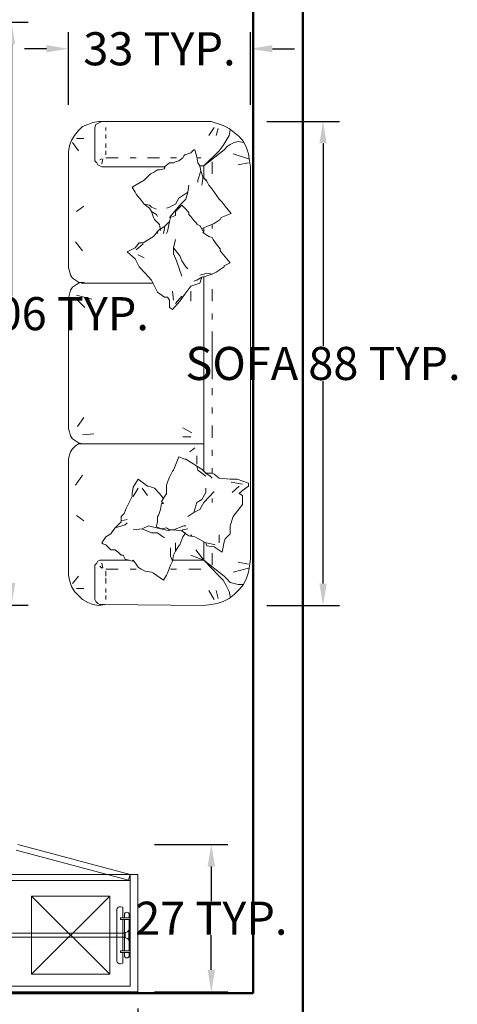
# Model space of a CAD drawing. Units: inches. Extents: x -466983 to 1020, y 324 to 318697.
# Tile 96 of 97: x 940 to 1020, y 827 to 1006. Entities that reach past the tile are written whole.
import ezdxf

# ---------------------------------------------------------------- set-up
doc = ezdxf.new("R2010")
doc.units = ezdxf.units.IN
doc.header["$MEASUREMENT"] = 0
for name, color, linetype, lineweight in [('A-ANNO-DIMS', 2, 'Continuous', 18), ('A-FURN', 8, 'Continuous', 18), ('A-WALL', 7, 'Continuous', 50)]:
    doc.layers.add(name, color=color, linetype=linetype, lineweight=lineweight)
doc.styles.get("Standard").update_dxf_attribs({"font": 'arial.ttf'})
doc.dimstyles.get("Standard").update_dxf_attribs({"dimtxt": 6, "dimasz": 4, "dimexe": 3, "dimexo": 3, "dimgap": 0.09, "dimtad": 0, "dimtih": 1, "dimtoh": 1, "dimdec": 1, "dimzin": 0, "dimdsep": 46, "dimlunit": 3, "dimtxsty": 'Standard', "dimcen": 0.09, "dimadec": 0, "dimazin": 0, "dimtfac": 1, "dimtdec": 1, "dimtofl": 0, "dimtmove": 0, "dimatfit": 3, "dimfxl": 1, "dimtolj": 1, "dimtzin": 0, "dimarcsym": 0})

# ---------------------------------------------------------------- blocks, each defined once
blk = doc.blocks.new('Wardrobe')
for p, q in [((2738.89, 1517.19, 0), (2738.89, 1543.9, 0)), ((2738.89, 1543.9, 0), (2850.18, 1543.9, 0)), ((2848.4, 1542.57, 0), (2740.67, 1542.57, 0)), ((2740.67, 1542.57, 0), (2740.67, 1517.19, 0)), ((2740.94, 1532.1, 0), (2740.67, 1532.1, 0)), ((2740.94, 1532.1, 0), (2740.67, 1532.1, 0)), ((2740.94, 1532.1, 0), (2740.94, 1529.88, 0)), ((2740.94, 1532.1, 0), (2740.94, 1529.88, 0)), ((2741.78, 1531.61, 0), (2741.78, 1530.37, 0)), ((2741.78, 1531.45, 0), (2792.53, 1531.45, 0)), ((2740.94, 1529.88, 0), (2740.67, 1529.88, 0)), ((2740.94, 1529.88, 0), (2740.67, 1529.88, 0)), ((2741.78, 1530.56, 0), (2792.53, 1530.56, 0)), ((2848.4, 1518.53, 0), (2740.67, 1518.53, 0)), ((2740.67, 1517.19, 0), (2741.02, 1518.48, 0)), ((2741.02, 1518.48, 0), (2766.6, 1511.65, 0)), ((2740.67, 1517.19, 0), (2738.89, 1517.19, 0)), ((2848.4, 1517.19, 0), (2740.67, 1517.19, 0)), ((2766.26, 1510.37, 0), (2740.67, 1517.19, 0))]:
    blk.add_line(p, q)
at = {"ltscale": 0.106667}
for p, q in [((2745.32, 1522.09, 0), (2763.13, 1539.9, 0)), ((2745.32, 1522.09, 0), (2745.32, 1539.9, 0)), ((2745.32, 1539.9, 0), (2763.13, 1539.9, 0)), ((2763.13, 1522.09, 0), (2745.32, 1539.9, 0)), ((2763.13, 1539.9, 0), (2763.13, 1522.09, 0)), ((2763.13, 1522.09, 0), (2745.32, 1522.09, 0))]:
    blk.add_line(p, q, dxfattribs=at)
at = {"ltscale": 0.02}
for p, q in [((2742.34, 1537.37, 0), (2742.84, 1537.5, 0)), ((2740.87, 1534.92, 0), (2740.87, 1535.62, 0)), ((2741.99, 1535.62, 0), (2741.99, 1534.92, 0)), ((2742.34, 1534.92, 0), (2742.34, 1537.37, 0)), ((2743.67, 1536.85, 0), (2743.67, 1525.18, 0)), ((2740.67, 1534.92, 0), (2742.84, 1534.92, 0)), ((2742.84, 1534.53, 0), (2740.67, 1534.53, 0)), ((2740.87, 1527.45, 0), (2740.87, 1534.53, 0)), ((2741.99, 1534.53, 0), (2741.99, 1527.45, 0)), ((2742.34, 1527.45, 0), (2742.34, 1534.53, 0)), ((2742.84, 1534.92, 0), (2742.84, 1534.53, 0)), ((2742.84, 1527.45, 0), (2740.67, 1527.45, 0)), ((2740.67, 1527.07, 0), (2742.84, 1527.07, 0)), ((2740.87, 1526.34, 0), (2740.87, 1527.07, 0)), ((2741.99, 1527.07, 0), (2741.99, 1526.34, 0)), ((2742.34, 1524.65, 0), (2742.34, 1527.07, 0)), ((2742.84, 1527.07, 0), (2742.84, 1527.45, 0)), ((2742.86, 1524.53, 0), (2742.34, 1524.65, 0))]:
    blk.add_line(p, q, dxfattribs=at)
for centre, radius, start, end in [((2743.01, 1536.85, 0), 0.668, 360, 104.1887), ((2741.43, 1535.62, 0), 0.556, 0, 180), ((2741.43, 1526.34, 0), 0.556, 180, 0), ((2743.01, 1525.18, 0), 0.668, 257.5257, 0)]:
    blk.add_arc(centre, radius, start, end, dxfattribs=at)
for centre, start, end in [((2741.78, 1532.59, 0), 209.9156, 269.9473), ((2741.78, 1532.59, 0), 209.9156, 269.9473), ((2741.78, 1529.39, 0), 90.0527, 150.0844)]:
    blk.add_arc(centre, 0.977, start, end)
blk = doc.blocks.new('sofa-36')
at = {"linetype": 'ByBlock'}
for p, q in [((-0.16, 0.87), (-0.135, 0.885)), ((-0.135, 0.885), (-0.16, 0.87)), ((-0.135, 0.885), (-0.105, 0.895)), ((-0.105, 0.895), (-0.135, 0.885)), ((-0.085, 0.85), (-0.12, 0.88)), ((-0.105, 0.895), (-0.08, 0.9)), ((-0.08, 0.9), (-0.105, 0.895)), ((-0.08, 0.9), (0.495, 0.9)), ((0.495, 0.9), (-0.08, 0.9)), ((0.495, 0.9), (0.515, 0.895)), ((0.515, 0.895), (0.495, 0.9)), ((0.515, 0.895), (0.53, 0.89)), ((0.53, 0.89), (0.515, 0.895)), ((0.53, 0.89), (0.545, 0.88)), ((0.545, 0.88), (0.53, 0.89)), ((0.545, 0.88), (0.56, 0.865)), ((0.56, 0.865), (0.545, 0.88)), ((0.585, 0.865), (0.595, 0.88)), ((0.585, 0.865), (0.595, 0.88)), ((0.595, 0.88), (0.61, 0.89)), ((0.595, 0.88), (0.61, 0.89)), ((0.61, 0.89), (0.63, 0.895)), ((0.61, 0.89), (0.63, 0.895)), ((0.63, 0.895), (0.645, 0.9)), ((0.63, 0.895), (0.645, 0.9)), ((0.645, 0.9), (0.87, 0.9)), ((0.87, 0.9), (0.645, 0.9)), ((0.87, 0.9), (1.29, 0.9)), ((1.29, 0.9), (0.87, 0.9)), ((1.29, 0.9), (1.31, 0.895)), ((1.31, 0.895), (1.29, 0.9)), ((1.31, 0.895), (1.33, 0.89)), ((1.33, 0.89), (1.31, 0.895)), ((1.33, 0.89), (1.345, 0.88)), ((1.345, 0.88), (1.33, 0.89)), ((1.345, 0.88), (1.355, 0.865)), ((1.355, 0.865), (1.345, 0.88)), ((1.38, 0.865), (1.39, 0.88)), ((1.38, 0.865), (1.39, 0.88)), ((1.39, 0.88), (1.405, 0.89)), ((1.39, 0.88), (1.405, 0.89)), ((1.405, 0.89), (1.425, 0.895)), ((1.405, 0.89), (1.425, 0.895)), ((1.425, 0.895), (1.44, 0.9)), ((1.425, 0.895), (1.44, 0.9)), ((1.44, 0.9), (2.015, 0.9)), ((2.015, 0.9), (1.44, 0.9)), ((2.015, 0.9), (2.045, 0.895)), ((2.045, 0.895), (2.015, 0.9)), ((2.02, 0.85), (2.06, 0.88)), ((2.045, 0.895), (2.07, 0.885)), ((2.07, 0.885), (2.045, 0.895)), ((2.07, 0.885), (2.095, 0.87)), ((2.095, 0.87), (2.07, 0.885)), ((-0.215, 0.805), (-0.2, 0.83)), ((-0.2, 0.83), (-0.215, 0.805)), ((-0.2, 0.83), (-0.18, 0.85)), ((-0.18, 0.85), (-0.2, 0.83)), ((-0.18, 0.85), (-0.16, 0.87)), ((-0.16, 0.87), (-0.18, 0.85)), ((-0.145, 0.825), (-0.145, 0.86)), ((0.19, 0.825), (0.215, 0.86)), ((0.415, 0.83), (0.365, 0.865)), ((0.56, 0.865), (0.57, 0.85)), ((0.57, 0.85), (0.56, 0.865)), ((0.57, 0.83), (0.575, 0.85)), ((0.57, 0.85), (0.57, 0.83)), ((0.57, 0.83), (0.57, 0.85)), ((0.57, 0.83), (0.575, 0.85)), ((0.57, 0.835), (0.57, 0.23)), ((0.57, 0.815), (0.57, 0.83)), ((0.57, 0.815), (0.57, 0.83)), ((0.575, 0.85), (0.585, 0.865)), ((0.575, 0.85), (0.585, 0.865)), ((0.615, 0.83), (0.62, 0.775)), ((0.655, 0.855), (0.7, 0.825)), ((1.28, 0.855), (1.245, 0.82)), ((1.305, 0.86), (1.285, 0.785)), ((1.355, 0.865), (1.365, 0.85)), ((1.365, 0.85), (1.355, 0.865)), ((1.365, 0.85), (1.3675, 0.84)), ((1.37, 0.83), (1.365, 0.85)), ((1.365, 0.83), (1.37, 0.85)), ((1.365, 0.835), (1.365, 0.48)), ((1.365, 0.815), (1.37, 0.83)), ((1.365, 0.815), (1.365, 0.83)), ((1.3675, 0.84), (1.37, 0.85)), ((1.37, 0.85), (1.38, 0.865)), ((1.37, 0.85), (1.38, 0.865)), ((1.525, 0.83), (1.57, 0.865)), ((1.745, 0.825), (1.72, 0.86)), ((2.08, 0.825), (2.08, 0.86)), ((2.095, 0.87), (2.12, 0.85)), ((2.12, 0.85), (2.095, 0.87)), ((2.12, 0.85), (2.14, 0.83)), ((2.14, 0.83), (2.12, 0.85)), ((2.14, 0.83), (2.15, 0.805)), ((2.15, 0.805), (2.14, 0.83)), ((-0.23, 0.75), (-0.225, 0.78)), ((-0.225, 0.78), (-0.23, 0.75)), ((-0.225, 0.78), (-0.215, 0.805)), ((-0.215, 0.805), (-0.225, 0.78)), ((2.15, 0.805), (2.16, 0.78)), ((2.16, 0.78), (2.15, 0.805)), ((2.16, 0.78), (2.165, 0.75)), ((2.165, 0.75), (2.16, 0.78)), ((-0.225, 0.72), (-0.23, 0.75)), ((-0.23, 0.75), (-0.225, 0.72)), ((-0.225, 0.745), (-0.22, 0.755)), ((-0.225, 0.735), (-0.225, 0.745)), ((-0.225, 0.72), (-0.225, 0.735)), ((-0.22, 0.755), (-0.21, 0.765)), ((-0.21, 0.765), (-0.2, 0.77)), ((-0.2, 0.77), (-0.19, 0.77)), ((-0.19, 0.77), (-0.175, 0.77)), ((-0.175, 0.77), (-0.055, 0.77)), ((-0.055, 0.77), (-0.04, 0.77)), ((-0.045, 0.735), (-0.035, 0.745)), ((-0.045, 0.73), (-0.02, 0.735)), ((-0.04, 0.77), (-0.03, 0.77)), ((-0.03, 0.77), (-0.02, 0.76)), ((-0.02, 0.76), (-0.01, 0.755)), ((-0.01, 0.755), (-0.005, 0.745)), ((-0.005, 0.745), (-0.005, 0.735)), ((-0.005, 0.735), (-0.005, 0.72)), ((0.08, 0.735), (0.075, 0.73)), ((0.11, 0.715), (0.08, 0.735)), ((1.94, 0.735), (1.945, 0.745)), ((1.94, 0.72), (1.94, 0.735)), ((1.945, 0.745), (1.95, 0.755)), ((1.95, 0.755), (1.96, 0.76)), ((1.98, 0.73), (1.955, 0.735)), ((1.96, 0.76), (1.97, 0.77)), ((1.97, 0.77), (1.98, 0.77)), ((1.98, 0.735), (1.975, 0.745)), ((1.98, 0.77), (1.99, 0.77)), ((1.99, 0.77), (2.115, 0.77)), ((2.115, 0.77), (2.125, 0.77)), ((2.125, 0.77), (2.135, 0.77)), ((2.135, 0.77), (2.15, 0.765)), ((2.15, 0.765), (2.155, 0.755)), ((2.155, 0.755), (2.16, 0.745)), ((2.16, 0.745), (2.165, 0.735)), ((2.165, 0.75), (2.165, 0.72)), ((2.165, 0.72), (2.165, 0.75)), ((2.165, 0.735), (2.165, 0.72)), ((-0.23, 0.23), (-0.225, 0.72)), ((-0.23, 0.23), (-0.225, 0.72)), ((-0.2, 0.715), (-0.18, 0.715)), ((-0.165, 0.715), (-0.145, 0.715)), ((-0.12, 0.715), (-0.095, 0.715)), ((-0.085, 0.715), (-0.06, 0.715)), ((-0.05, 0.715), (-0.05, 0.655)), ((-0.005, 0.72), (-0.005, 0.6)), ((0.07, 0.715), (0.045, 0.69)), ((0.045, 0.69), (0.045, 0.68)), ((0.075, 0.73), (0.07, 0.715)), ((0.125, 0.69), (0.11, 0.715)), ((0.14, 0.68), (0.125, 0.69)), ((1.94, 0.42), (1.94, 0.72)), ((1.985, 0.715), (1.985, 0.655)), ((2.02, 0.715), (2, 0.715)), ((2.055, 0.715), (2.035, 0.715)), ((2.1, 0.715), (2.08, 0.715)), ((2.135, 0.715), (2.12, 0.715)), ((2.165, 0.72), (2.165, 0.23)), ((2.165, 0.72), (2.165, 0.23)), ((0.035, 0.655), (0.02, 0.64)), ((0.02, 0.64), (0.02, 0.63)), ((0.045, 0.67), (0.035, 0.655)), ((0.045, 0.68), (0.045, 0.67)), ((0.155, 0.67), (0.14, 0.68)), ((0.155, 0.67), (0.17, 0.62)), ((0.185, 0.64), (0.155, 0.67)), ((0.185, 0.64), (0.21, 0.64)), ((0.19, 0.64), (0.185, 0.64)), ((0.195, 0.61), (0.19, 0.64)), ((0.21, 0.64), (0.225, 0.625)), ((-0.05, 0.595), (-0.05, 0.565)), ((0, 0.62), (-0.01, 0.585)), ((-0.01, 0.585), (-0.005, 0.58)), ((0.02, 0.63), (0, 0.62)), ((0.17, 0.62), (0.18, 0.61)), ((0.225, 0.625), (0.25, 0.615)), ((0.235, 0.62), (0.235, 0.62)), ((0.25, 0.615), (0.31, 0.585)), ((0.31, 0.585), (0.325, 0.585)), ((0.325, 0.585), (0.355, 0.58)), ((1.52, 0.61), (1.485, 0.57)), ((1.54, 0.57), (1.52, 0.61)), ((1.815, 0.57), (1.84, 0.585)), ((1.84, 0.585), (1.875, 0.525)), ((1.985, 0.595), (1.985, 0.565)), ((-0.05, 0.54), (-0.06, 0.52)), ((-0.04, 0.555), (-0.05, 0.54)), ((-0.025, 0.565), (-0.04, 0.555)), ((-0.005, 0.58), (-0.025, 0.565)), ((0.15, 0.535), (0.145, 0.58)), ((0.35, 0.555), (0.31, 0.58)), ((0.355, 0.58), (0.395, 0.555)), ((0.395, 0.555), (0.36, 0.51)), ((1.445, 0.55), (1.415, 0.52)), ((1.475, 0.565), (1.445, 0.55)), ((1.485, 0.57), (1.475, 0.565)), ((1.505, 0.555), (1.49, 0.525)), ((1.53, 0.565), (1.56, 0.53)), ((1.565, 0.55), (1.54, 0.57)), ((1.565, 0.53), (1.565, 0.55)), ((1.755, 0.525), (1.775, 0.54)), ((1.775, 0.54), (1.805, 0.565)), ((1.805, 0.565), (1.815, 0.57)), ((-0.065, 0.49), (-0.07, 0.48)), ((-0.06, 0.52), (-0.065, 0.49)), ((0.15, 0.535), (0.13, 0.49)), ((0.13, 0.49), (0.13, 0.46)), ((0.165, 0.505), (0.15, 0.535)), ((0.155, 0.465), (0.165, 0.505)), ((0.35, 0.535), (0.315, 0.51)), ((0.36, 0.505), (0.35, 0.475)), ((0.36, 0.51), (0.36, 0.505)), ((1.38, 0.49), (1.32, 0.46)), ((1.415, 0.52), (1.38, 0.49)), ((1.595, 0.48), (1.565, 0.53)), ((1.72, 0.49), (1.69, 0.48)), ((1.705, 0.465), (1.72, 0.49)), ((1.72, 0.49), (1.735, 0.5)), ((1.74, 0.49), (1.73, 0.465)), ((1.735, 0.5), (1.755, 0.525)), ((1.75, 0.5), (1.74, 0.49)), ((1.755, 0.525), (1.75, 0.5)), ((1.875, 0.525), (1.88, 0.52)), ((1.88, 0.52), (1.905, 0.495)), ((1.905, 0.495), (1.915, 0.475)), ((1.985, 0.45), (1.985, 0.51)), ((-0.07, 0.48), (-0.105, 0.43)), ((0.115, 0.44), (0.105, 0.425)), ((0.13, 0.46), (0.115, 0.44)), ((0.14, 0.4), (0.155, 0.465)), ((0.16, 0.465), (0.15, 0.44)), ((0.15, 0.44), (0.155, 0.415)), ((0.165, 0.465), (0.16, 0.465)), ((0.185, 0.46), (0.165, 0.465)), ((0.21, 0.46), (0.185, 0.46)), ((0.215, 0.455), (0.21, 0.46)), ((0.23, 0.45), (0.215, 0.455)), ((0.245, 0.445), (0.23, 0.45)), ((0.275, 0.44), (0.245, 0.445)), ((0.275, 0.43), (0.275, 0.44)), ((0.285, 0.44), (0.275, 0.43)), ((0.325, 0.415), (0.285, 0.44)), ((0.325, 0.45), (0.3, 0.43)), ((0.35, 0.475), (0.325, 0.45)), ((1.32, 0.46), (1.295, 0.425)), ((1.62, 0.46), (1.595, 0.48)), ((1.615, 0.46), (1.61, 0.46)), ((1.63, 0.45), (1.62, 0.46)), ((1.655, 0.45), (1.625, 0.445)), ((1.645, 0.425), (1.63, 0.45)), ((1.68, 0.475), (1.655, 0.45)), ((1.69, 0.48), (1.68, 0.475)), ((1.695, 0.46), (1.705, 0.465)), ((1.915, 0.475), (1.925, 0.46)), ((1.925, 0.46), (1.925, 0.45)), ((1.925, 0.45), (1.93, 0.425)), ((-0.105, 0.43), (-0.08, 0.415)), ((-0.08, 0.415), (-0.07, 0.41)), ((-0.07, 0.41), (-0.03, 0.395)), ((-0.05, 0.365), (-0.05, 0.395)), ((-0.03, 0.395), (-0.01, 0.385)), ((-0.01, 0.385), (0.015, 0.395)), ((0.015, 0.395), (0.03, 0.395)), ((0.03, 0.395), (0.055, 0.395)), ((0.155, 0.415), (0.145, 0.4)), ((0.145, 0.4), (0.145, 0.38)), ((0.32, 0.415), (0.325, 0.415)), ((0.355, 0.415), (0.32, 0.415)), ((0.365, 0.415), (0.355, 0.415)), ((0.38, 0.41), (0.365, 0.415)), ((0.405, 0.4), (0.38, 0.41)), ((0.435, 0.385), (0.405, 0.4)), ((1.245, 0.4), (1.235, 0.385)), ((1.28, 0.4), (1.245, 0.4)), ((1.295, 0.41), (1.28, 0.4)), ((1.295, 0.425), (1.295, 0.41)), ((1.61, 0.43), (1.635, 0.425)), ((1.62, 0.41), (1.61, 0.415)), ((1.67, 0.4), (1.62, 0.41)), ((1.635, 0.425), (1.645, 0.425)), ((1.645, 0.425), (1.67, 0.4)), ((1.67, 0.4), (1.69, 0.395)), ((1.69, 0.4), (1.75, 0.35)), ((1.69, 0.395), (1.7, 0.37)), ((1.74, 0.4), (1.735, 0.415)), ((1.755, 0.37), (1.74, 0.4)), ((1.93, 0.425), (1.94, 0.425)), ((1.94, 0.425), (1.96, 0.4)), ((1.96, 0.4), (1.96, 0.38)), ((1.985, 0.365), (1.985, 0.395)), ((-0.01, 0.385), (0.02, 0.38)), ((-0.005, 0.385), (-0.005, 0.23)), ((0.02, 0.38), (0.04, 0.37)), ((0.04, 0.37), (0.065, 0.355)), ((0.04, 0.37), (0.065, 0.37)), ((0.065, 0.37), (0.08, 0.37)), ((0.065, 0.355), (0.07, 0.35)), ((0.07, 0.35), (0.11, 0.335)), ((0.145, 0.38), (0.14, 0.34)), ((0.145, 0.38), (0.165, 0.33)), ((0.44, 0.38), (0.435, 0.385)), ((0.505, 0.355), (0.44, 0.38)), ((0.495, 0.325), (0.505, 0.355)), ((1.235, 0.385), (1.275, 0.35)), ((1.265, 0.37), (1.3, 0.34)), ((1.275, 0.35), (1.31, 0.325)), ((1.28, 0.38), (1.325, 0.385)), ((1.4, 0.34), (1.475, 0.365)), ((1.475, 0.365), (1.51, 0.38)), ((1.5, 0.35), (1.475, 0.34)), ((1.54, 0.38), (1.5, 0.35)), ((1.51, 0.38), (1.54, 0.38)), ((1.54, 0.38), (1.58, 0.37)), ((1.7, 0.37), (1.72, 0.37)), ((1.72, 0.37), (1.75, 0.34)), ((1.75, 0.35), (1.78, 0.32)), ((1.785, 0.355), (1.755, 0.37)), ((1.815, 0.31), (1.785, 0.355)), ((1.96, 0.38), (1.965, 0.37)), ((1.965, 0.37), (1.97, 0.355)), ((1.97, 0.355), (1.985, 0.335)), ((-0.05, 0.245), (-0.05, 0.305)), ((0.02, 0.295), (-0.005, 0.23)), ((0.11, 0.335), (0.13, 0.32)), ((0.115, 0.305), (0.11, 0.275)), ((0.125, 0.32), (0.115, 0.305)), ((0.12, 0.295), (0.115, 0.29)), ((0.14, 0.34), (0.125, 0.32)), ((0.14, 0.34), (0.145, 0.335)), ((0.145, 0.335), (0.15, 0.31)), ((0.165, 0.33), (0.165, 0.32)), ((0.23, 0.28), (0.21, 0.31)), ((0.47, 0.28), (0.495, 0.32)), ((0.495, 0.32), (0.495, 0.325)), ((0.55, 0.275), (0.53, 0.3)), ((0.605, 0.295), (0.605, 0.335)), ((0.625, 0.29), (0.65, 0.335)), ((1.325, 0.295), (1.275, 0.295)), ((1.31, 0.325), (1.35, 0.295)), ((1.35, 0.295), (1.36, 0.265)), ((1.445, 0.32), (1.435, 0.31)), ((1.475, 0.34), (1.445, 0.32)), ((1.695, 0.295), (1.675, 0.28)), ((1.705, 0.305), (1.695, 0.295)), ((1.715, 0.305), (1.705, 0.305)), ((1.735, 0.325), (1.715, 0.305)), ((1.745, 0.335), (1.735, 0.325)), ((1.75, 0.34), (1.745, 0.335)), ((1.78, 0.32), (1.815, 0.31)), ((1.815, 0.31), (1.85, 0.305)), ((1.985, 0.335), (1.995, 0.33)), ((1.995, 0.33), (2, 0.325)), ((2, 0.325), (2.01, 0.295)), ((2.01, 0.295), (2.025, 0.28)), ((0.045, 0.27), (-0.005, 0.23)), ((0.11, 0.275), (0.08, 0.22)), ((0.23, 0.28), (0.28, 0.265)), ((0.245, 0.25), (0.23, 0.28)), ((0.28, 0.23), (0.245, 0.25)), ((0.28, 0.265), (0.295, 0.24)), ((0.425, 0.24), (0.44, 0.26)), ((0.44, 0.26), (0.46, 0.265)), ((0.445, 0.24), (0.46, 0.265)), ((0.46, 0.265), (0.47, 0.28)), ((0.51, 0.265), (0.47, 0.265)), ((1.36, 0.265), (1.365, 0.25)), ((1.365, 0.25), (1.395, 0.24)), ((1.38, 0.265), (1.375, 0.28)), ((1.395, 0.24), (1.38, 0.265)), ((1.41, 0.23), (1.405, 0.25)), ((1.65, 0.25), (1.615, 0.23)), ((1.655, 0.265), (1.65, 0.25)), ((1.66, 0.265), (1.655, 0.265)), ((1.675, 0.28), (1.66, 0.265)), ((1.875, 0.26), (1.865, 0.26)), ((1.92, 0.245), (1.875, 0.26)), ((1.92, 0.245), (1.89, 0.235)), ((1.945, 0.25), (1.92, 0.245)), ((1.96, 0.26), (1.945, 0.25)), ((1.945, 0.25), (1.945, 0.23)), ((1.99, 0.265), (1.96, 0.26)), ((1.985, 0.245), (1.985, 0.26)), ((2.025, 0.275), (1.99, 0.265)), ((2.025, 0.28), (2.025, 0.275)), ((-0.225, 0.195), (-0.23, 0.23)), ((-0.225, 0.195), (-0.23, 0.23)), ((-0.22, 0.165), (-0.225, 0.195)), ((-0.22, 0.165), (-0.225, 0.195)), ((-0.2, 0.18), (-0.155, 0.205)), ((-0.005, 0.23), (-0.085, 0.13)), ((-0.005, 0.23), (-0.085, 0.155)), ((0.085, 0.23), (-0.005, 0.23)), ((0.065, 0.215), (0.06, 0.18)), ((0.08, 0.22), (0.065, 0.215)), ((0.07, 0.175), (0.08, 0.215)), ((0.335, 0.18), (0.28, 0.23)), ((0.295, 0.24), (0.33, 0.22)), ((0.33, 0.22), (0.35, 0.22)), ((0.41, 0.2), (0.4, 0.19)), ((0.41, 0.22), (0.425, 0.24)), ((0.425, 0.22), (0.41, 0.2)), ((0.425, 0.22), (0.445, 0.24)), ((0.425, 0.19), (0.425, 0.22)), ((0.435, 0.23), (0.87, 0.23)), ((1.395, 0.23), (0.87, 0.23)), ((1.4, 0.22), (1.395, 0.24)), ((1.41, 0.19), (1.4, 0.22)), ((1.415, 0.215), (1.41, 0.23)), ((1.41, 0.19), (1.415, 0.215)), ((1.595, 0.205), (1.59, 0.19)), ((1.615, 0.235), (1.595, 0.205)), ((1.615, 0.23), (1.615, 0.235)), ((1.615, 0.23), (1.615, 0.23)), ((1.64, 0.23), (1.62, 0.23)), ((1.645, 0.215), (1.635, 0.24)), ((1.66, 0.18), (1.645, 0.215)), ((1.85, 0.205), (1.83, 0.19)), ((1.845, 0.2), (1.845, 0.2)), ((1.88, 0.235), (1.85, 0.24)), ((1.87, 0.215), (1.85, 0.205)), ((1.89, 0.235), (1.87, 0.215)), ((1.87, 0.215), (1.88, 0.22)), ((1.89, 0.235), (1.88, 0.235)), ((1.885, 0.23), (1.945, 0.23)), ((1.945, 0.23), (2.025, 0.13)), ((1.945, 0.23), (2.02, 0.155)), ((2.135, 0.18), (2.095, 0.205)), ((2.165, 0.195), (2.155, 0.165)), ((2.165, 0.195), (2.155, 0.165)), ((2.165, 0.23), (2.165, 0.195)), ((2.165, 0.23), (2.165, 0.195)), ((-0.21, 0.135), (-0.22, 0.165)), ((-0.21, 0.135), (-0.22, 0.165)), ((-0.155, 0.17), (-0.195, 0.16)), ((-0.085, 0.155), (-0.105, 0.135)), ((-0.03, 0.19), (0.03, 0.19)), ((0.06, 0.18), (0.035, 0.14)), ((0.08, 0.155), (0.12, 0.155)), ((0.28, 0.19), (0.3, 0.19)), ((0.395, 0.1), (0.4, 0.155)), ((0.4, 0.155), (0.42, 0.18)), ((0.42, 0.18), (0.425, 0.19)), ((0.45, 0.19), (0.425, 0.19)), ((0.54, 0.19), (0.51, 0.19)), ((0.6, 0.19), (0.66, 0.19)), ((0.72, 0.19), (0.75, 0.19)), ((0.81, 0.19), (0.845, 0.19)), ((1.125, 0.19), (0.89, 0.19)), ((1.215, 0.19), (1.185, 0.19)), ((1.335, 0.19), (1.275, 0.19)), ((1.42, 0.17), (1.41, 0.19)), ((1.445, 0.13), (1.42, 0.17)), ((1.525, 0.15), (1.465, 0.1)), ((1.535, 0.15), (1.525, 0.15)), ((1.56, 0.17), (1.535, 0.15)), ((1.58, 0.185), (1.56, 0.17)), ((1.59, 0.19), (1.58, 0.185)), ((1.655, 0.19), (1.635, 0.19)), ((1.68, 0.15), (1.66, 0.18)), ((1.69, 0.145), (1.68, 0.15)), ((1.78, 0.155), (1.765, 0.14)), ((1.83, 0.19), (1.78, 0.155)), ((1.965, 0.19), (1.905, 0.19)), ((2.02, 0.155), (2.045, 0.135)), ((2.095, 0.17), (2.13, 0.16)), ((2.155, 0.165), (2.145, 0.135)), ((2.155, 0.165), (2.145, 0.135)), ((-0.195, 0.105), (-0.21, 0.135)), ((-0.195, 0.105), (-0.21, 0.135)), ((-0.175, 0.08), (-0.195, 0.105)), ((-0.175, 0.08), (-0.195, 0.105)), ((-0.16, 0.105), (-0.185, 0.1)), ((-0.13, 0.12), (-0.16, 0.105)), ((-0.105, 0.135), (-0.13, 0.12)), ((-0.115, 0.1), (-0.12, 0.08)), ((-0.1, 0.115), (-0.115, 0.1)), ((-0.085, 0.13), (-0.1, 0.115)), ((0.035, 0.14), (0.085, 0.13)), ((0.085, 0.13), (0.1, 0.125)), ((0.1, 0.125), (0.125, 0.1)), ((0.125, 0.1), (0.165, 0.1)), ((0.165, 0.1), (0.21, 0.085)), ((0.395, 0.065), (0.395, 0.1)), ((1.45, 0.13), (1.445, 0.13)), ((1.465, 0.1), (1.45, 0.13)), ((1.71, 0.095), (1.69, 0.145)), ((1.745, 0.125), (1.71, 0.095)), ((1.765, 0.14), (1.745, 0.125)), ((2.025, 0.13), (2.04, 0.115)), ((2.04, 0.115), (2.05, 0.1)), ((2.045, 0.135), (2.07, 0.12)), ((2.05, 0.1), (2.06, 0.08)), ((2.07, 0.12), (2.095, 0.105)), ((2.095, 0.105), (2.125, 0.1)), ((2.13, 0.105), (2.11, 0.08)), ((2.13, 0.105), (2.11, 0.08)), ((2.145, 0.135), (2.13, 0.105)), ((2.145, 0.135), (2.13, 0.105)), ((-0.15, 0.055), (-0.175, 0.08)), ((-0.15, 0.055), (-0.175, 0.08)), ((-0.125, 0.035), (-0.15, 0.055)), ((-0.125, 0.035), (-0.15, 0.055)), ((-0.12, 0.08), (-0.125, 0.06)), ((-0.125, 0.06), (-0.125, 0.035)), ((-0.045, 0.01), (-0.065, 0.085)), ((-0.015, 0.06), (-0.025, 0.01)), ((0.21, 0.085), (0.27, 0.04)), ((0.315, 0.04), (0.325, 0.055)), ((0.325, 0.055), (0.34, 0.04)), ((0.36, 0.055), (0.33, 0.09)), ((0.37, 0.04), (0.38, 0.095)), ((0.375, 0.01), (0.395, 0.065)), ((1.95, 0.06), (1.96, 0.01)), ((1.98, 0.01), (2.005, 0.085)), ((2.06, 0.08), (2.065, 0.06)), ((2.065, 0.06), (2.06, 0.035)), ((2.09, 0.055), (2.065, 0.035)), ((2.09, 0.055), (2.065, 0.035)), ((2.11, 0.08), (2.09, 0.055)), ((2.11, 0.08), (2.09, 0.055)), ((-0.095, 0.02), (-0.125, 0.035)), ((-0.095, 0.02), (-0.125, 0.035)), ((-0.065, 0.01), (-0.095, 0.02)), ((-0.065, 0.01), (-0.095, 0.02)), ((-0.035, 0.005), (-0.065, 0.01)), ((-0.035, 0.005), (-0.065, 0.01)), ((0, 0), (-0.035, 0.005)), ((0, 0), (-0.035, 0.005)), ((1.94, 0), (0, 0)), ((1.94, 0), (0, 0)), ((0.27, 0.04), (0.315, 0.04)), ((0.34, 0.04), (0.36, 0.01)), ((0.36, 0.01), (0.375, 0.01)), ((1.97, 0.005), (1.94, 0)), ((1.97, 0.005), (1.94, 0)), ((2.005, 0.01), (1.97, 0.005)), ((2.005, 0.01), (1.97, 0.005)), ((2.035, 0.02), (2.005, 0.01)), ((2.035, 0.02), (2.005, 0.01)), ((2.065, 0.035), (2.035, 0.02)), ((2.065, 0.035), (2.035, 0.02))]:
    blk.add_line(p, q, dxfattribs=at)
blk = doc.blocks.new('*D73')
at = {"layer": 'A-ANNO-DIMS', "color": 0, "lineweight": -2, "transparency": 16777216}
for p, q in [((926.13, 1005.06), (942, 1005.06)), ((939, 1001.06), (939, 955.34)), ((939, 903.32), (939, 949.04)), ((926.13, 899.32), (942, 899.32))]:
    blk.add_line(p, q, dxfattribs=at)
at = {"layer": 'A-ANNO-DIMS', "color": 0, "transparency": 16777216}
for points in [[(938.33, 1001.06), (939.66, 1001.06), (939, 1005.06)], [(938.33, 903.32), (939.66, 903.32), (939, 899.32)]]:
    blk.add_solid(points, dxfattribs=at)
at = {"layer": 'Defpoints', "color": 0, "transparency": 16777216}
for p in [(923.13, 1005.06), (939, 1005.06), (923.13, 899.32)]:
    blk.add_point(p, dxfattribs=at)
at = {"layer": 'A-ANNO-DIMS', "color": 0, "transparency": 16777216, "insert": (939, 952.19), "char_height": 6, "attachment_point": 5}
blk.add_mtext('\\A1;BED 106 TYP.', dxfattribs=at)
blk = doc.blocks.new('*D81')
at = {"layer": 'A-ANNO-DIMS', "color": 0, "lineweight": -2, "transparency": 16777216}
for p, q in [((873.26, 826.19), (873.26, 812.89)), ((961.93, 826.19), (961.93, 812.89)), ((869.26, 815.89), (865.26, 815.89)), ((965.93, 815.89), (969.93, 815.89))]:
    blk.add_line(p, q, dxfattribs=at)
at = {"layer": 'A-ANNO-DIMS', "color": 0, "transparency": 16777216}
for points in [[(869.26, 816.56), (869.26, 815.23), (873.26, 815.89)], [(965.93, 816.56), (965.93, 815.23), (961.93, 815.89)]]:
    blk.add_solid(points, dxfattribs=at)
at = {"layer": 'Defpoints', "color": 0, "transparency": 16777216}
for p in [(873.26, 829.19), (961.93, 829.19), (873.26, 815.89)]:
    blk.add_point(p, dxfattribs=at)
at = {"layer": 'A-ANNO-DIMS', "color": 0, "transparency": 16777216, "insert": (917.59, 815.89), "char_height": 6, "attachment_point": 5}
blk.add_mtext('\\A1;WARDROBE 89 TYP.', dxfattribs=at)
blk = doc.blocks.new('*D82')
at = {"layer": 'A-ANNO-DIMS', "color": 0, "lineweight": -2, "transparency": 16777216}
for p, q in [((964.93, 855.92), (978.23, 855.92)), ((975.23, 851.92), (975.23, 845.66)), ((975.23, 833.19), (975.23, 839.45)), ((964.93, 829.19), (978.23, 829.19))]:
    blk.add_line(p, q, dxfattribs=at)
at = {"layer": 'A-ANNO-DIMS', "color": 0, "transparency": 16777216}
for points in [[(974.56, 851.92), (975.9, 851.92), (975.23, 855.92)], [(974.56, 833.19), (975.9, 833.19), (975.23, 829.19)]]:
    blk.add_solid(points, dxfattribs=at)
at = {"layer": 'Defpoints', "color": 0, "transparency": 16777216}
for p in [(961.93, 855.92), (961.93, 829.19), (975.23, 829.19)]:
    blk.add_point(p, dxfattribs=at)
at = {"layer": 'A-ANNO-DIMS', "color": 0, "transparency": 16777216, "insert": (975.23, 842.55), "char_height": 6, "attachment_point": 5}
blk.add_mtext('\\A1;27 TYP.', dxfattribs=at)
blk = doc.blocks.new('*D87')
at = {"layer": 'A-ANNO-DIMS', "color": 0, "lineweight": -2, "transparency": 16777216}
for p, q in [((985.33, 987.06), (998.5, 987.06)), ((995.5, 983.06), (995.5, 946.35)), ((995.5, 903.25), (995.5, 939.96)), ((985.33, 899.25), (998.5, 899.25))]:
    blk.add_line(p, q, dxfattribs=at)
at = {"layer": 'A-ANNO-DIMS', "color": 0, "transparency": 16777216}
for points in [[(994.83, 983.06), (996.17, 983.06), (995.5, 987.06)], [(994.83, 903.25), (996.17, 903.25), (995.5, 899.25)]]:
    blk.add_solid(points, dxfattribs=at)
at = {"layer": 'Defpoints', "color": 0, "transparency": 16777216}
for p in [(982.33, 987.06), (995.5, 987.06), (982.33, 899.25)]:
    blk.add_point(p, dxfattribs=at)
at = {"layer": 'A-ANNO-DIMS', "color": 0, "transparency": 16777216, "insert": (995.5, 943.16), "char_height": 6, "attachment_point": 5}
blk.add_mtext('\\A1;SOFA 88 TYP.', dxfattribs=at)
blk = doc.blocks.new('*D88')
at = {"layer": 'A-ANNO-DIMS', "color": 0, "lineweight": -2, "transparency": 16777216}
for p, q in [((949.33, 990.06), (949.33, 1003.23)), ((982.33, 990.06), (982.33, 1003.23)), ((945.33, 1000.23), (941.33, 1000.23)), ((986.33, 1000.23), (990.33, 1000.23))]:
    blk.add_line(p, q, dxfattribs=at)
at = {"layer": 'A-ANNO-DIMS', "color": 0, "transparency": 16777216}
for points in [[(945.33, 1000.9), (945.33, 999.57), (949.33, 1000.23)], [(986.33, 1000.9), (986.33, 999.57), (982.33, 1000.23)]]:
    blk.add_solid(points, dxfattribs=at)
at = {"layer": 'Defpoints', "color": 0, "transparency": 16777216}
for p in [(949.33, 1000.23), (949.33, 987.06), (982.33, 987.06)]:
    blk.add_point(p, dxfattribs=at)
at = {"layer": 'A-ANNO-DIMS', "color": 0, "transparency": 16777216, "insert": (965.83, 1000.23), "char_height": 6, "attachment_point": 5}
blk.add_mtext('\\A1;33 TYP.', dxfattribs=at)

msp = doc.modelspace()

# ---------------------------------------------------------------- linework, layer by layer
at = {"layer": 'A-WALL'}
for p, q in [((991.81, 1084.94), (991.81, 364.94)), ((982.81, 1075.94), (982.81, 828.94)), ((982.81, 828.94), (813.81, 828.94))]:
    msp.add_line(p, q, dxfattribs=at)

# ---------------------------------------------------------------- block references
at = {"layer": 'A-FURN'}
for name, p, xscale, yscale, zscale, rotation in [('sofa-36', (982.33, 907.68), 36.66436083614781, 36.66436083614781, 36.66436083614781, 89.99999999999999), ('Wardrobe', (3144.16, 2059.31, 0), 0.7967580954171016, 0.7967580954171016, 0.7967580954171016, 180)]:
    msp.add_blockref(name, p, dxfattribs=dict(at, xscale=xscale, yscale=yscale, zscale=zscale, rotation=rotation))

# ---------------------------------------------------------------- dimensions: what is measured, and where the dimension line sits
at = {"layer": 'A-ANNO-DIMS'}
for base, p1, p2, angle, text, picture, middle in [((949.33, 1000.23), (982.33, 987.06), (949.33, 987.06), 180, '<> TYP.', '*D88', (965.83, 1000.23)), ((939, 1005.06), (923.13, 899.32), (923.13, 1005.06), 90, 'BED <> TYP.', '*D73', (939, 952.19)), ((995.5, 987.06), (982.33, 899.25), (982.33, 987.06), 90, 'SOFA <> TYP.', '*D87', (995.5, 943.16)), ((975.23, 829.19), (961.93, 855.92), (961.93, 829.19), 270, '<> TYP.', '*D82', (975.23, 842.55)), ((873.26, 815.89), (961.93, 829.19), (873.26, 829.19), 180, 'WARDROBE <> TYP.', '*D81', (917.59, 815.89))]:
    dim = msp.add_linear_dim(base=base, p1=p1, p2=p2, angle=angle, text=text, dimstyle='Standard', override={"dimdec": 0, "dimlfac": 1, "dimrnd": 0, "dimzin": 0, "dimdsep": 46, "dimlunit": 2}, dxfattribs=at)
    dim.commit()
    dim.dimension.update_dxf_attribs({"geometry": picture, "text_midpoint": middle})

doc.saveas('drawing.dxf')
